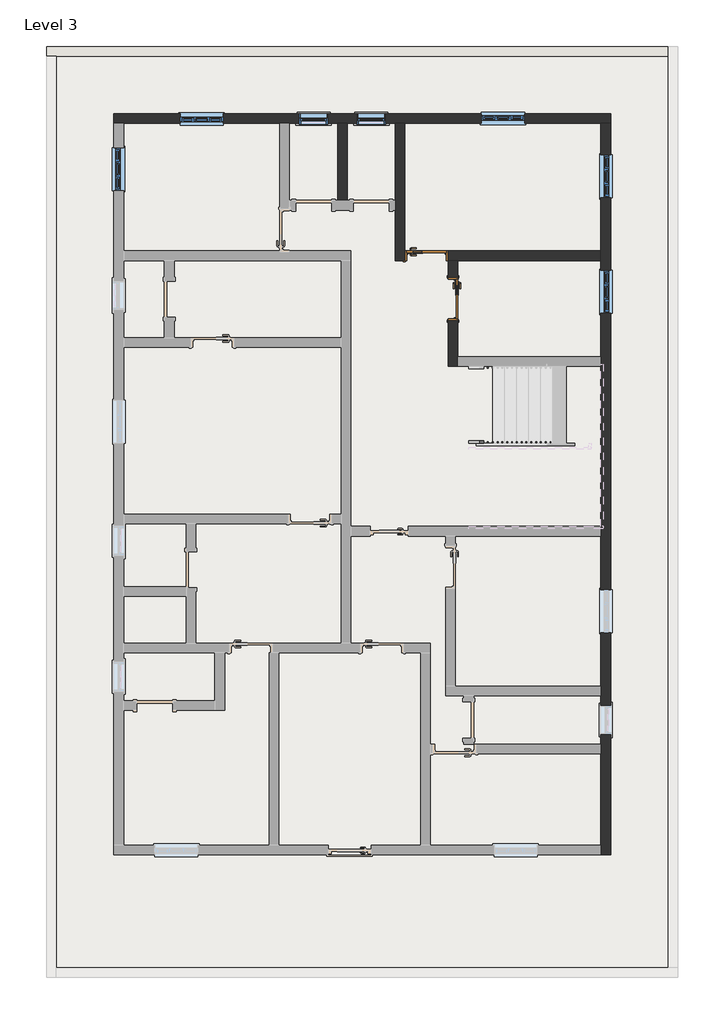
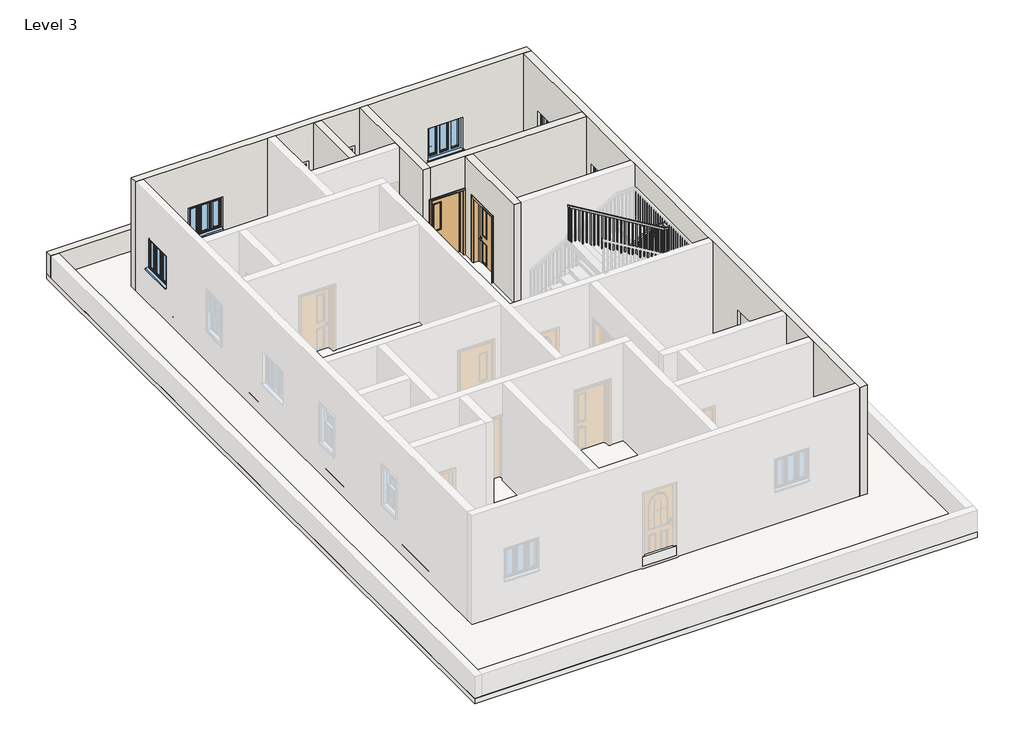
# One storey, part 2 of 3: 7 walls, 7 windows, 2 doors, 2 slabs, 1 railing, 1 roof.
"""IFC4 building model written with IfcOpenShell, lengths in millimetres."""

from ifc_helpers import new_model, si_unit, frame, origin, place, context, project, spatial, polyline, outline, extrude, faceted_brep, transform, mapped, element, save
from components import door_aa1d4bf3, window_679d2811, windows_tpl_w_glazing_bars_910x910mm_9d987a72

model = new_model("IFC4")

# Units and contexts
model_context = context("Model", 3, world=origin())
ifc_project = project(units=[si_unit("LENGTHUNIT", "METRE", prefix="MILLI")], contexts=[model_context])

# Site, building, storey
site = spatial("IfcSite", under=ifc_project)
building = spatial("IfcBuilding", under=site)
storey = spatial("IfcBuildingStorey", under=building, Name="Level 3", Elevation=6096.0)

# Doors
placement = place(None, origin())
door_shape = door_aa1d4bf3(model_context)
element("IfcDoor", 1, ObjectType="Doors_IntSgl_3 : 7'-3\"", at=placement, inside=storey, context=model_context, shape_type="MappedRepresentation", body=[
    mapped(door_shape, transform((-7303.1711241, 14069.3344295, 6096.0), x_axis=(1.0, 0.0, 0.0), y_axis=(0.0, 1.0, 0.0), z_axis=(0.0, 0.0, 1.0))),
])
element("IfcDoor", 2, ObjectType="Doors_IntSgl_3 : 7'-3\"", at=placement, inside=storey, context=model_context, shape_type="MappedRepresentation", body=[
    mapped(door_shape, transform((-6744.3711241, 13154.9344295, 6096.0), x_axis=(0.0, -1.0, 0.0), y_axis=(1.0, 0.0, 0.0), z_axis=(0.0, 0.0, 1.0))),
])

# Railing
element("IfcRailing", 3, ObjectType="Handrail - Rectangular", at=placement, inside=storey, context=model_context, shape_type="SolidModel", body=[
    faceted_brep([(-6414.1711241, 10157.7344295, 7162.8), (-6414.1711241, 10157.7344295, 7103.5575287), (-6414.1711241, 10106.9344295, 7103.5575287), (-6414.1711241, 10106.9344295, 7162.8), (-4128.1711241, 10157.7344295, 8534.4), (-4114.1003386, 10157.7344295, 8483.6), (-4114.1003386, 10106.9344295, 8483.6), (-4128.1711241, 10106.9344295, 8534.4), (-3772.5711241, 10157.7344295, 8534.4), (-3772.5711241, 10157.7344295, 8483.6), (-3823.3711241, 10106.9344295, 8483.6), (-3823.3711241, 10106.9344295, 8534.4), (-3772.5711241, 9929.1344295, 8534.4), (-3772.5711241, 9929.1344295, 8483.6), (-3823.3711241, 9979.9344295, 8483.6), (-3823.3711241, 9979.9344295, 8534.4), (-3874.1711241, 9929.1344295, 8534.4), (-3888.2419095, 9929.1344295, 8483.6), (-3888.2419095, 9979.9344295, 8483.6), (-3874.1711241, 9979.9344295, 8534.4), (-6414.1711241, 9929.1344295, 10058.4), (-6414.1711241, 9979.9344295, 10058.4), (-6414.1711241, 9979.9344295, 9999.1575287), (-6414.1711241, 9929.1344295, 9999.1575287)], [[[0, 1, 2, 3]], [[1, 0, 4, 5]], [[2, 1, 5, 6]], [[3, 2, 6, 7]], [[0, 3, 7, 4]], [[5, 4, 8, 9]], [[6, 5, 9, 10]], [[7, 6, 10, 11]], [[4, 7, 11, 8]], [[9, 8, 12, 13]], [[10, 9, 13, 14]], [[11, 10, 14, 15]], [[8, 11, 15, 12]], [[13, 12, 16, 17]], [[14, 13, 17, 18]], [[15, 14, 18, 19]], [[12, 15, 19, 16]], [[20, 21, 22, 23]], [[17, 16, 20, 23]], [[18, 17, 23, 22]], [[19, 18, 22, 21]], [[16, 19, 21, 20]]]),
    extrude(outline(polyline([(9947.7225287, -6328.4461241), (9959.1525287, -6347.4961241), (8991.6, -6347.4961241), (8991.6, -6328.4461241), (9947.7225287, -6328.4461241)])), frame((0.0, 9945.0094295, 0.0), z_axis=(0.0, 1.0, 0.0), x_axis=(0.0, 0.0, 1.0)), (0.0, 0.0, 1.0), 19.05),
    extrude(outline(polyline([(9886.7625287, -6226.8461241), (9898.1925287, -6245.8961241), (8991.6, -6245.8961241), (8991.6, -6226.8461241), (9886.7625287, -6226.8461241)])), frame((0.0, 9945.0094295, 0.0), z_axis=(0.0, 1.0, 0.0), x_axis=(0.0, 0.0, 1.0)), (0.0, 0.0, 1.0), 19.05),
    extrude(outline(polyline([(9825.8025287, -6125.2461241), (9837.2325287, -6144.2961241), (8839.2, -6144.2961241), (8839.2, -6125.2461241), (9825.8025287, -6125.2461241)])), frame((0.0, 9945.0094295, 0.0), z_axis=(0.0, 1.0, 0.0), x_axis=(0.0, 0.0, 1.0)), (0.0, 0.0, 1.0), 19.05),
    extrude(outline(polyline([(9764.8425287, -6023.6461241), (9776.2725287, -6042.6961241), (8839.2, -6042.6961241), (8839.2, -6023.6461241), (9764.8425287, -6023.6461241)])), frame((0.0, 9945.0094295, 0.0), z_axis=(0.0, 1.0, 0.0), x_axis=(0.0, 0.0, 1.0)), (0.0, 0.0, 1.0), 19.05),
    extrude(outline(polyline([(9703.8825287, -5922.0461241), (9715.3125287, -5941.0961241), (8839.2, -5941.0961241), (8839.2, -5922.0461241), (9703.8825287, -5922.0461241)])), frame((0.0, 9945.0094295, 0.0), z_axis=(0.0, 1.0, 0.0), x_axis=(0.0, 0.0, 1.0)), (0.0, 0.0, 1.0), 19.05),
    extrude(outline(polyline([(9642.9225287, -5820.4461241), (9654.3525287, -5839.4961241), (8686.8, -5839.4961241), (8686.8, -5820.4461241), (9642.9225287, -5820.4461241)])), frame((0.0, 9945.0094295, 0.0), z_axis=(0.0, 1.0, 0.0), x_axis=(0.0, 0.0, 1.0)), (0.0, 0.0, 1.0), 19.05),
    extrude(outline(polyline([(9581.9625287, -5718.8461241), (9593.3925287, -5737.8961241), (8686.8, -5737.8961241), (8686.8, -5718.8461241), (9581.9625287, -5718.8461241)])), frame((0.0, 9945.0094295, 0.0), z_axis=(0.0, 1.0, 0.0), x_axis=(0.0, 0.0, 1.0)), (0.0, 0.0, 1.0), 19.05),
    extrude(outline(polyline([(9521.0025287, -5617.2461241), (9532.4325287, -5636.2961241), (8534.4, -5636.2961241), (8534.4, -5617.2461241), (9521.0025287, -5617.2461241)])), frame((0.0, 9945.0094295, 0.0), z_axis=(0.0, 1.0, 0.0), x_axis=(0.0, 0.0, 1.0)), (0.0, 0.0, 1.0), 19.05),
    extrude(outline(polyline([(9460.0425287, -5515.6461241), (9471.4725287, -5534.6961241), (8534.4, -5534.6961241), (8534.4, -5515.6461241), (9460.0425287, -5515.6461241)])), frame((0.0, 9945.0094295, 0.0), z_axis=(0.0, 1.0, 0.0), x_axis=(0.0, 0.0, 1.0)), (0.0, 0.0, 1.0), 19.05),
    extrude(outline(polyline([(9399.0825287, -5414.0461241), (9410.5125287, -5433.0961241), (8534.4, -5433.0961241), (8534.4, -5414.0461241), (9399.0825287, -5414.0461241)])), frame((0.0, 9945.0094295, 0.0), z_axis=(0.0, 1.0, 0.0), x_axis=(0.0, 0.0, 1.0)), (0.0, 0.0, 1.0), 19.05),
    extrude(outline(polyline([(9338.1225287, -5312.4461241), (9349.5525287, -5331.4961241), (8382.0, -5331.4961241), (8382.0, -5312.4461241), (9338.1225287, -5312.4461241)])), frame((0.0, 9945.0094295, 0.0), z_axis=(0.0, 1.0, 0.0), x_axis=(0.0, 0.0, 1.0)), (0.0, 0.0, 1.0), 19.05),
    extrude(outline(polyline([(9277.1625287, -5210.8461241), (9288.5925287, -5229.8961241), (8382.0, -5229.8961241), (8382.0, -5210.8461241), (9277.1625287, -5210.8461241)])), frame((0.0, 9945.0094295, 0.0), z_axis=(0.0, 1.0, 0.0), x_axis=(0.0, 0.0, 1.0)), (0.0, 0.0, 1.0), 19.05),
    extrude(outline(polyline([(9216.2025287, -5109.2461241), (9227.6325287, -5128.2961241), (8229.6, -5128.2961241), (8229.6, -5109.2461241), (9216.2025287, -5109.2461241)])), frame((0.0, 9945.0094295, 0.0), z_axis=(0.0, 1.0, 0.0), x_axis=(0.0, 0.0, 1.0)), (0.0, 0.0, 1.0), 19.05),
    extrude(outline(polyline([(9155.2425287, -5007.6461241), (9166.6725287, -5026.6961241), (8229.6, -5026.6961241), (8229.6, -5007.6461241), (9155.2425287, -5007.6461241)])), frame((0.0, 9945.0094295, 0.0), z_axis=(0.0, 1.0, 0.0), x_axis=(0.0, 0.0, 1.0)), (0.0, 0.0, 1.0), 19.05),
    extrude(outline(polyline([(9094.2825287, -4906.0461241), (9105.7125287, -4925.0961241), (8229.6, -4925.0961241), (8229.6, -4906.0461241), (9094.2825287, -4906.0461241)])), frame((0.0, 9945.0094295, 0.0), z_axis=(0.0, 1.0, 0.0), x_axis=(0.0, 0.0, 1.0)), (0.0, 0.0, 1.0), 19.05),
    extrude(outline(polyline([(9033.3225287, -4804.4461241), (9044.7525287, -4823.4961241), (8077.2, -4823.4961241), (8077.2, -4804.4461241), (9033.3225287, -4804.4461241)])), frame((0.0, 9945.0094295, 0.0), z_axis=(0.0, 1.0, 0.0), x_axis=(0.0, 0.0, 1.0)), (0.0, 0.0, 1.0), 19.05),
    extrude(outline(polyline([(8972.3625287, -4702.8461241), (8983.7925287, -4721.8961241), (8077.2, -4721.8961241), (8077.2, -4702.8461241), (8972.3625287, -4702.8461241)])), frame((0.0, 9945.0094295, 0.0), z_axis=(0.0, 1.0, 0.0), x_axis=(0.0, 0.0, 1.0)), (0.0, 0.0, 1.0), 19.05),
    extrude(outline(polyline([(8911.4025287, -4601.2461241), (8922.8325287, -4620.2961241), (7924.8, -4620.2961241), (7924.8, -4601.2461241), (8911.4025287, -4601.2461241)])), frame((0.0, 9945.0094295, 0.0), z_axis=(0.0, 1.0, 0.0), x_axis=(0.0, 0.0, 1.0)), (0.0, 0.0, 1.0), 19.05),
    extrude(outline(polyline([(8850.4425287, -4499.6461241), (8861.8725287, -4518.6961241), (7924.8, -4518.6961241), (7924.8, -4499.6461241), (8850.4425287, -4499.6461241)])), frame((0.0, 9945.0094295, 0.0), z_axis=(0.0, 1.0, 0.0), x_axis=(0.0, 0.0, 1.0)), (0.0, 0.0, 1.0), 19.05),
    extrude(outline(polyline([(8789.4825287, -4398.0461241), (8800.9125287, -4417.0961241), (7924.8, -4417.0961241), (7924.8, -4398.0461241), (8789.4825287, -4398.0461241)])), frame((0.0, 9945.0094295, 0.0), z_axis=(0.0, 1.0, 0.0), x_axis=(0.0, 0.0, 1.0)), (0.0, 0.0, 1.0), 19.05),
    extrude(outline(polyline([(8728.5225287, -4296.4461241), (8739.9525287, -4315.4961241), (7772.4, -4315.4961241), (7772.4, -4296.4461241), (8728.5225287, -4296.4461241)])), frame((0.0, 9945.0094295, 0.0), z_axis=(0.0, 1.0, 0.0), x_axis=(0.0, 0.0, 1.0)), (0.0, 0.0, 1.0), 19.05),
    extrude(outline(polyline([(8667.5625287, -4194.8461241), (8678.9925287, -4213.8961241), (7772.4, -4213.8961241), (7772.4, -4194.8461241), (8667.5625287, -4194.8461241)])), frame((0.0, 9945.0094295, 0.0), z_axis=(0.0, 1.0, 0.0), x_axis=(0.0, 0.0, 1.0)), (0.0, 0.0, 1.0), 19.05),
    extrude(outline(polyline([(8606.6025287, -4093.2461241), (8618.0325287, -4112.2961241), (7620.0, -4112.2961241), (7620.0, -4093.2461241), (8606.6025287, -4093.2461241)])), frame((0.0, 9945.0094295, 0.0), z_axis=(0.0, 1.0, 0.0), x_axis=(0.0, 0.0, 1.0)), (0.0, 0.0, 1.0), 19.05),
    extrude(outline(polyline([(8545.6425287, -3991.6461241), (8557.0725287, -4010.6961241), (7620.0, -4010.6961241), (7620.0, -3991.6461241), (8545.6425287, -3991.6461241)])), frame((0.0, 9945.0094295, 0.0), z_axis=(0.0, 1.0, 0.0), x_axis=(0.0, 0.0, 1.0)), (0.0, 0.0, 1.0), 19.05),
    extrude(outline(polyline([(8484.6825287, -3890.0461241), (8496.1125287, -3909.0961241), (7620.0, -3909.0961241), (7620.0, -3890.0461241), (8484.6825287, -3890.0461241)])), frame((0.0, 9945.0094295, 0.0), z_axis=(0.0, 1.0, 0.0), x_axis=(0.0, 0.0, 1.0)), (0.0, 0.0, 1.0), 19.05),
    extrude(outline(polyline([(-3807.4961241, 10040.2594295), (-3788.4461241, 10040.2594295), (-3788.4461241, 10021.2094295), (-3807.4961241, 10021.2094295), (-3807.4961241, 10040.2594295)])), frame((0.0, 0.0, 7620.0), z_axis=(0.0, 0.0, 1.0), x_axis=(1.0, 0.0, 0.0)), (0.0, 0.0, 1.0), 863.6),
    extrude(outline(polyline([(-3883.6961241, 10122.8094295), (-3883.6961241, 10141.8594295), (-3864.6461241, 10141.8594295), (-3864.6461241, 10122.8094295), (-3883.6961241, 10122.8094295)])), frame((0.0, 0.0, 7620.0), z_axis=(0.0, 0.0, 1.0), x_axis=(1.0, 0.0, 0.0)), (0.0, 0.0, 1.0), 863.6),
    extrude(outline(polyline([(-3985.2961241, 10122.8094295), (-3985.2961241, 10141.8594295), (-3966.2461241, 10141.8594295), (-3966.2461241, 10122.8094295), (-3985.2961241, 10122.8094295)])), frame((0.0, 0.0, 7620.0), z_axis=(0.0, 0.0, 1.0), x_axis=(1.0, 0.0, 0.0)), (0.0, 0.0, 1.0), 863.6),
    extrude(outline(polyline([(-4086.8961241, 10122.8094295), (-4086.8961241, 10141.8594295), (-4067.8461241, 10141.8594295), (-4067.8461241, 10122.8094295), (-4086.8961241, 10122.8094295)])), frame((0.0, 0.0, 7620.0), z_axis=(0.0, 0.0, 1.0), x_axis=(1.0, 0.0, 0.0)), (0.0, 0.0, 1.0), 863.6),
    extrude(outline(polyline([(8450.3925287, -4169.4461241), (8438.9625287, -4188.4961241), (7467.6, -4188.4961241), (7467.6, -4169.4461241), (8450.3925287, -4169.4461241)])), frame((0.0, 10122.8094295, 0.0), z_axis=(0.0, 1.0, 0.0), x_axis=(0.0, 0.0, 1.0)), (0.0, 0.0, 1.0), 19.05),
    extrude(outline(polyline([(8389.4325287, -4271.0461241), (8378.0025287, -4290.0961241), (7467.6, -4290.0961241), (7467.6, -4271.0461241), (8389.4325287, -4271.0461241)])), frame((0.0, 10122.8094295, 0.0), z_axis=(0.0, 1.0, 0.0), x_axis=(0.0, 0.0, 1.0)), (0.0, 0.0, 1.0), 19.05),
    extrude(outline(polyline([(8328.4725287, -4372.6461241), (8317.0425287, -4391.6961241), (7467.6, -4391.6961241), (7467.6, -4372.6461241), (8328.4725287, -4372.6461241)])), frame((0.0, 10122.8094295, 0.0), z_axis=(0.0, 1.0, 0.0), x_axis=(0.0, 0.0, 1.0)), (0.0, 0.0, 1.0), 19.05),
    extrude(outline(polyline([(8267.5125287, -4474.2461241), (8256.0825287, -4493.2961241), (7315.2, -4493.2961241), (7315.2, -4474.2461241), (8267.5125287, -4474.2461241)])), frame((0.0, 10122.8094295, 0.0), z_axis=(0.0, 1.0, 0.0), x_axis=(0.0, 0.0, 1.0)), (0.0, 0.0, 1.0), 19.05),
    extrude(outline(polyline([(8206.5525287, -4575.8461241), (8195.1225287, -4594.8961241), (7315.2, -4594.8961241), (7315.2, -4575.8461241), (8206.5525287, -4575.8461241)])), frame((0.0, 10122.8094295, 0.0), z_axis=(0.0, 1.0, 0.0), x_axis=(0.0, 0.0, 1.0)), (0.0, 0.0, 1.0), 19.05),
    extrude(outline(polyline([(8145.5925287, -4677.4461241), (8134.1625287, -4696.4961241), (7162.8, -4696.4961241), (7162.8, -4677.4461241), (8145.5925287, -4677.4461241)])), frame((0.0, 10122.8094295, 0.0), z_axis=(0.0, 1.0, 0.0), x_axis=(0.0, 0.0, 1.0)), (0.0, 0.0, 1.0), 19.05),
    extrude(outline(polyline([(8084.6325287, -4779.0461241), (8073.2025287, -4798.0961241), (7162.8, -4798.0961241), (7162.8, -4779.0461241), (8084.6325287, -4779.0461241)])), frame((0.0, 10122.8094295, 0.0), z_axis=(0.0, 1.0, 0.0), x_axis=(0.0, 0.0, 1.0)), (0.0, 0.0, 1.0), 19.05),
    extrude(outline(polyline([(8023.6725287, -4880.6461241), (8012.2425287, -4899.6961241), (7162.8, -4899.6961241), (7162.8, -4880.6461241), (8023.6725287, -4880.6461241)])), frame((0.0, 10122.8094295, 0.0), z_axis=(0.0, 1.0, 0.0), x_axis=(0.0, 0.0, 1.0)), (0.0, 0.0, 1.0), 19.05),
    extrude(outline(polyline([(7962.7125287, -4982.2461241), (7951.2825287, -5001.2961241), (7010.4, -5001.2961241), (7010.4, -4982.2461241), (7962.7125287, -4982.2461241)])), frame((0.0, 10122.8094295, 0.0), z_axis=(0.0, 1.0, 0.0), x_axis=(0.0, 0.0, 1.0)), (0.0, 0.0, 1.0), 19.05),
    extrude(outline(polyline([(7901.7525287, -5083.8461241), (7890.3225287, -5102.8961241), (7010.4, -5102.8961241), (7010.4, -5083.8461241), (7901.7525287, -5083.8461241)])), frame((0.0, 10122.8094295, 0.0), z_axis=(0.0, 1.0, 0.0), x_axis=(0.0, 0.0, 1.0)), (0.0, 0.0, 1.0), 19.05),
    extrude(outline(polyline([(7840.7925287, -5185.4461241), (7829.3625287, -5204.4961241), (6858.0, -5204.4961241), (6858.0, -5185.4461241), (7840.7925287, -5185.4461241)])), frame((0.0, 10122.8094295, 0.0), z_axis=(0.0, 1.0, 0.0), x_axis=(0.0, 0.0, 1.0)), (0.0, 0.0, 1.0), 19.05),
    extrude(outline(polyline([(7779.8325287, -5287.0461241), (7768.4025287, -5306.0961241), (6858.0, -5306.0961241), (6858.0, -5287.0461241), (7779.8325287, -5287.0461241)])), frame((0.0, 10122.8094295, 0.0), z_axis=(0.0, 1.0, 0.0), x_axis=(0.0, 0.0, 1.0)), (0.0, 0.0, 1.0), 19.05),
    extrude(outline(polyline([(7718.8725287, -5388.6461241), (7707.4425287, -5407.6961241), (6858.0, -5407.6961241), (6858.0, -5388.6461241), (7718.8725287, -5388.6461241)])), frame((0.0, 10122.8094295, 0.0), z_axis=(0.0, 1.0, 0.0), x_axis=(0.0, 0.0, 1.0)), (0.0, 0.0, 1.0), 19.05),
    extrude(outline(polyline([(7657.9125287, -5490.2461241), (7646.4825287, -5509.2961241), (6705.6, -5509.2961241), (6705.6, -5490.2461241), (7657.9125287, -5490.2461241)])), frame((0.0, 10122.8094295, 0.0), z_axis=(0.0, 1.0, 0.0), x_axis=(0.0, 0.0, 1.0)), (0.0, 0.0, 1.0), 19.05),
    extrude(outline(polyline([(7596.9525287, -5591.8461241), (7585.5225287, -5610.8961241), (6705.6, -5610.8961241), (6705.6, -5591.8461241), (7596.9525287, -5591.8461241)])), frame((0.0, 10122.8094295, 0.0), z_axis=(0.0, 1.0, 0.0), x_axis=(0.0, 0.0, 1.0)), (0.0, 0.0, 1.0), 19.05),
    extrude(outline(polyline([(7535.9925287, -5693.4461241), (7524.5625287, -5712.4961241), (6553.2, -5712.4961241), (6553.2, -5693.4461241), (7535.9925287, -5693.4461241)])), frame((0.0, 10122.8094295, 0.0), z_axis=(0.0, 1.0, 0.0), x_axis=(0.0, 0.0, 1.0)), (0.0, 0.0, 1.0), 19.05),
    extrude(outline(polyline([(7475.0325287, -5795.0461241), (7463.6025287, -5814.0961241), (6553.2, -5814.0961241), (6553.2, -5795.0461241), (7475.0325287, -5795.0461241)])), frame((0.0, 10122.8094295, 0.0), z_axis=(0.0, 1.0, 0.0), x_axis=(0.0, 0.0, 1.0)), (0.0, 0.0, 1.0), 19.05),
    extrude(outline(polyline([(7414.0725287, -5896.6461241), (7402.6425287, -5915.6961241), (6553.2, -5915.6961241), (6553.2, -5896.6461241), (7414.0725287, -5896.6461241)])), frame((0.0, 10122.8094295, 0.0), z_axis=(0.0, 1.0, 0.0), x_axis=(0.0, 0.0, 1.0)), (0.0, 0.0, 1.0), 19.05),
    extrude(outline(polyline([(7353.1125287, -5998.2461241), (7341.6825287, -6017.2961241), (6400.8, -6017.2961241), (6400.8, -5998.2461241), (7353.1125287, -5998.2461241)])), frame((0.0, 10122.8094295, 0.0), z_axis=(0.0, 1.0, 0.0), x_axis=(0.0, 0.0, 1.0)), (0.0, 0.0, 1.0), 19.05),
    extrude(outline(polyline([(7292.1525287, -6099.8461241), (7280.7225287, -6118.8961241), (6400.8, -6118.8961241), (6400.8, -6099.8461241), (7292.1525287, -6099.8461241)])), frame((0.0, 10122.8094295, 0.0), z_axis=(0.0, 1.0, 0.0), x_axis=(0.0, 0.0, 1.0)), (0.0, 0.0, 1.0), 19.05),
    extrude(outline(polyline([(7231.1925287, -6201.4461241), (7219.7625287, -6220.4961241), (6248.4, -6220.4961241), (6248.4, -6201.4461241), (7231.1925287, -6201.4461241)])), frame((0.0, 10122.8094295, 0.0), z_axis=(0.0, 1.0, 0.0), x_axis=(0.0, 0.0, 1.0)), (0.0, 0.0, 1.0), 19.05),
    extrude(outline(polyline([(7170.2325287, -6303.0461241), (7158.8025287, -6322.0961241), (6248.4, -6322.0961241), (6248.4, -6303.0461241), (7170.2325287, -6303.0461241)])), frame((0.0, 10122.8094295, 0.0), z_axis=(0.0, 1.0, 0.0), x_axis=(0.0, 0.0, 1.0)), (0.0, 0.0, 1.0), 19.05),
    extrude(outline(polyline([(-3807.4961241, 9964.0594295), (-3788.4461241, 9964.0594295), (-3788.4461241, 9945.0094295), (-3807.4961241, 9945.0094295), (-3807.4961241, 9964.0594295)])), frame((0.0, 0.0, 7620.0), z_axis=(0.0, 0.0, 1.0), x_axis=(1.0, 0.0, 0.0)), (0.0, 0.0, 1.0), 863.6),
    extrude(outline(polyline([(-3807.4961241, 10122.8094295), (-3807.4961241, 10141.8594295), (-3788.4461241, 10141.8594295), (-3788.4461241, 10122.8094295), (-3807.4961241, 10122.8094295)])), frame((0.0, 0.0, 7620.0), z_axis=(0.0, 0.0, 1.0), x_axis=(1.0, 0.0, 0.0)), (0.0, 0.0, 1.0), 863.6),
    extrude(outline(polyline([(9987.7275287, -6395.1211241), (9999.1575287, -6414.1711241), (8991.6, -6414.1711241), (8991.6, -6395.1211241), (9987.7275287, -6395.1211241)])), frame((0.0, 9945.0094295, 0.0), z_axis=(0.0, 1.0, 0.0), x_axis=(0.0, 0.0, 1.0)), (0.0, 0.0, 1.0), 19.05),
    extrude(outline(polyline([(7114.9875287, -6395.1211241), (7103.5575287, -6414.1711241), (6248.4, -6414.1711241), (6248.4, -6395.1211241), (7114.9875287, -6395.1211241)])), frame((0.0, 10122.8094295, 0.0), z_axis=(0.0, 1.0, 0.0), x_axis=(0.0, 0.0, 1.0)), (0.0, 0.0, 1.0), 19.05),
])

# Roof
element("IfcRoof", 4, ObjectType="Generic - 12\"", at=placement, inside=storey, context=model_context, shape_type="SweptSolid", body=[
    extrude(outline(polyline([(-13907.1711241, 17066.5344295), (-3416.9711241, 17066.5344295), (-3416.9711241, 1420.1344295), (-13907.1711241, 1420.1344295), (-13907.1711241, 17066.5344295)])), frame((0.0, 0.0, 6096.0), z_axis=(0.0, 0.0, 1.0), x_axis=(1.0, 0.0, 0.0)), (0.0, 0.0, 1.0), 304.8),
])

# Slabs
element("IfcSlab", 5, ObjectType="Generic - 12\"", at=placement, inside=storey, context=model_context, shape_type="SweptSolid", body=[
    extrude(outline(polyline([(-1994.5711241, 18488.2009778), (-1994.5711241, -1171.3990222), (-15329.5711241, -1171.3990222), (-15329.5711241, 18488.2009778), (-1994.5711241, 18488.2009778)])), frame((0.0, 0.0, 5943.6), z_axis=(0.0, 0.0, 1.0), x_axis=(1.0, 0.0, 0.0)), (0.0, 0.0, 1.0), 152.4),
])
element("IfcSlab", 6, ObjectType="Generic - 12\" 2", at=placement, inside=storey, context=model_context, shape_type="SweptSolid", body=[
    extrude(outline(polyline([(-3416.9711241, 17066.5344295), (-3416.9711241, 1420.1344295), (-13907.1711241, 1420.1344295), (-13907.1711241, 17066.5344295), (-3416.9711241, 17066.5344295)])), frame((0.0, 0.0, 5943.6), z_axis=(0.0, 0.0, 1.0), x_axis=(1.0, 0.0, 0.0)), (0.0, 0.0, 1.0), 152.4),
])

# Walls
element("IfcWall", 7, ObjectType="Generic -4.5\" p", at=placement, inside=storey, context=model_context, shape_type="SweptSolid", body=[
    extrude(outline(polyline([(-9182.7711241, 15237.7344295), (-9182.7711241, 16863.3344295), (-8979.5711241, 16863.3344295), (-8979.5711241, 15237.7344295), (-9182.7711241, 15237.7344295)])), frame((0.0, 0.0, 6096.0), z_axis=(0.0, 0.0, 1.0), x_axis=(1.0, 0.0, 0.0)), (0.0, 0.0, 1.0), 3048.0),
])
element("IfcWall", 8, ObjectType="Generic -4.5\" p", at=placement, inside=storey, context=model_context, shape_type="Brep", body=[
    faceted_brep([(-7963.5711241, 16863.3344295, 6096.0), (-7963.5711241, 15237.7344295, 6096.0), (-7963.5711241, 15034.5344295, 6096.0), (-7963.5711241, 13967.7344295, 6096.0), (-7963.5711241, 13967.7344295, 9144.0), (-7963.5711241, 15034.5344295, 9144.0), (-7963.5711241, 15237.7344295, 9144.0), (-7963.5711241, 16863.3344295, 9144.0), (-7760.3711241, 16863.3344295, 6096.0), (-7760.3711241, 16863.3344295, 9144.0), (-7760.3711241, 14170.9344295, 9144.0), (-7760.3711241, 13967.7344295, 9144.0), (-7760.3711241, 13967.7344295, 8229.6), (-7760.3711241, 13967.7344295, 6096.0)], [[[0, 1, 2, 3, 4, 5, 6, 7]], [[8, 9, 10, 11, 12, 13]], [[3, 2, 1, 0, 8, 13]], [[7, 6, 5, 4, 11, 10, 9]], [[0, 7, 9, 8]], [[4, 3, 13, 12, 11]]]),
])
element("IfcWall", 9, ObjectType="Generic -4.5\" p", at=placement, inside=storey, context=model_context, shape_type="Brep", body=[
    faceted_brep([(-7760.3711241, 14170.9344295, 9144.0), (-3620.1711241, 14170.9344295, 9144.0), (-3620.1711241, 14170.9344295, 6096.0), (-6845.9711241, 14170.9344295, 6096.0), (-6845.9711241, 14170.9344295, 8229.6), (-7760.3711241, 14170.9344295, 8229.6), (-3620.1711241, 13967.7344295, 9144.0), (-6642.7711241, 13967.7344295, 9144.0), (-6845.9711241, 13967.7344295, 9144.0), (-7760.3711241, 13967.7344295, 9144.0), (-7760.3711241, 13967.7344295, 8229.6), (-6845.9711241, 13967.7344295, 8229.6), (-6845.9711241, 13967.7344295, 6096.0), (-6642.7711241, 13967.7344295, 6096.0), (-3620.1711241, 13967.7344295, 6096.0)], [[[0, 1, 2, 3, 4, 5]], [[6, 7, 8, 9, 10, 11, 12, 13, 14]], [[2, 14, 13, 12, 3]], [[1, 0, 9, 8, 7, 6]], [[9, 0, 5, 10]], [[2, 1, 6, 14]], [[11, 4, 3, 12]], [[4, 11, 10, 5]]]),
])
element("IfcWall", 10, ObjectType="Generic -4.5\" p", at=placement, inside=storey, context=model_context, shape_type="Brep", body=[
    faceted_brep([(-6845.9711241, 11732.5344295, 9144.0), (-6845.9711241, 13967.7344295, 9144.0), (-6845.9711241, 13967.7344295, 8229.6), (-6845.9711241, 13967.7344295, 6096.0), (-6845.9711241, 13612.1344295, 6096.0), (-6845.9711241, 13612.1344295, 8229.6), (-6845.9711241, 12697.7344295, 8229.6), (-6845.9711241, 12697.7344295, 6096.0), (-6845.9711241, 11732.5344295, 6096.0), (-6642.7711241, 13967.7344295, 9144.0), (-6642.7711241, 11935.7344295, 9144.0), (-6642.7711241, 11732.5344295, 9144.0), (-6642.7711241, 11732.5344295, 6096.0), (-6642.7711241, 11935.7344295, 6096.0), (-6642.7711241, 12697.7344295, 6096.0), (-6642.7711241, 12697.7344295, 8229.6), (-6642.7711241, 13612.1344295, 8229.6), (-6642.7711241, 13612.1344295, 6096.0), (-6642.7711241, 13967.7344295, 6096.0)], [[[0, 1, 2, 3, 4, 5, 6, 7, 8]], [[9, 10, 11, 12, 13, 14, 15, 16, 17, 18]], [[3, 18, 17, 4]], [[12, 8, 7, 14, 13]], [[1, 0, 11, 10, 9]], [[3, 2, 1, 9, 18]], [[0, 8, 12, 11]], [[6, 15, 14, 7]], [[15, 6, 5, 16]], [[16, 5, 4, 17]]]),
])
element("IfcWall", 11, ObjectType="Generic -4.5\" p", at=placement, inside=storey, context=model_context, shape_type="Brep", body=[
    faceted_brep([(-15329.5711241, 18285.0009778, 6096.0), (-15126.3711241, 18285.0009778, 6096.0), (-2197.7711241, 18285.0009778, 6096.0), (-2197.7711241, 18285.0009778, 6705.6), (-15126.3711241, 18285.0009778, 6705.6), (-15329.5711241, 18285.0009778, 6705.6), (-15329.5711241, 18488.2009778, 6096.0), (-15329.5711241, 18488.2009778, 6705.6), (-2197.7711241, 18488.2009778, 6705.6), (-2197.7711241, 18488.2009778, 6096.0)], [[[0, 1, 2, 3, 4, 5]], [[6, 7, 8, 9]], [[2, 1, 0, 6, 9]], [[5, 4, 3, 8, 7]], [[0, 5, 7, 6]], [[3, 2, 9, 8]]]),
])
element("IfcWall", 12, ObjectType="Generic -9\" w", at=placement, inside=storey, context=model_context, shape_type="Brep", body=[
    faceted_brep([(-13907.1711241, 16863.3344295, 6096.0), (-13703.9711241, 16863.3344295, 6096.0), (-10401.9711241, 16863.3344295, 6096.0), (-10198.7711241, 16863.3344295, 6096.0), (-9182.7711241, 16863.3344295, 6096.0), (-8979.5711241, 16863.3344295, 6096.0), (-7963.5711241, 16863.3344295, 6096.0), (-7760.3711241, 16863.3344295, 6096.0), (-3620.1711241, 16863.3344295, 6096.0), (-3416.9711241, 16863.3344295, 6096.0), (-3416.9711241, 16863.3344295, 9144.0), (-3620.1711241, 16863.3344295, 9144.0), (-7760.3711241, 16863.3344295, 9144.0), (-7963.5711241, 16863.3344295, 9144.0), (-8979.5711241, 16863.3344295, 9144.0), (-9182.7711241, 16863.3344295, 9144.0), (-10198.7711241, 16863.3344295, 9144.0), (-10401.9711241, 16863.3344295, 9144.0), (-13703.9711241, 16863.3344295, 9144.0), (-13907.1711241, 16863.3344295, 9144.0), (-11597.9711241, 16863.3344295, 7920.4), (-11597.9711241, 16863.3344295, 7010.4), (-12507.9711241, 16863.3344295, 7010.4), (-12507.9711241, 16863.3344295, 7920.4), (-6145.2711241, 16863.3344295, 7920.4), (-5235.2711241, 16863.3344295, 7920.4), (-5235.2711241, 16863.3344295, 7010.4), (-6145.2711241, 16863.3344295, 7010.4), (-9385.9711241, 16863.3344295, 8077.2), (-9385.9711241, 16863.3344295, 7010.4), (-9995.5711241, 16863.3344295, 7010.4), (-9995.5711241, 16863.3344295, 8077.2), (-8166.7711241, 16863.3344295, 8077.2), (-8166.7711241, 16863.3344295, 7010.4), (-8776.3711241, 16863.3344295, 7010.4), (-8776.3711241, 16863.3344295, 8077.2), (-13907.1711241, 17066.5344295, 6096.0), (-13907.1711241, 17066.5344295, 9144.0), (-3416.9711241, 17066.5344295, 9144.0), (-3416.9711241, 17066.5344295, 6096.0), (-11597.9711241, 17066.5344295, 7920.4), (-12507.9711241, 17066.5344295, 7920.4), (-12507.9711241, 17066.5344295, 7010.4), (-11597.9711241, 17066.5344295, 7010.4), (-6145.2711241, 17066.5344295, 7920.4), (-6145.2711241, 17066.5344295, 7010.4), (-5235.2711241, 17066.5344295, 7010.4), (-5235.2711241, 17066.5344295, 7920.4), (-9385.9711241, 17066.5344295, 8077.2), (-9995.5711241, 17066.5344295, 8077.2), (-9995.5711241, 17066.5344295, 7010.4), (-9385.9711241, 17066.5344295, 7010.4), (-8166.7711241, 17066.5344295, 8077.2), (-8776.3711241, 17066.5344295, 8077.2), (-8776.3711241, 17066.5344295, 7010.4), (-8166.7711241, 17066.5344295, 7010.4)], [[[0, 1, 2, 3, 4, 5, 6, 7, 8, 9, 10, 11, 12, 13, 14, 15, 16, 17, 18, 19], [20, 21, 22, 23], [24, 25, 26, 27], [28, 29, 30, 31], [32, 33, 34, 35]], [[36, 37, 38, 39], [40, 41, 42, 43], [44, 45, 46, 47], [48, 49, 50, 51], [52, 53, 54, 55]], [[9, 8, 7, 6, 5, 4, 3, 2, 1, 0, 36, 39]], [[19, 18, 17, 16, 15, 14, 13, 12, 11, 10, 38, 37]], [[10, 9, 39, 38]], [[0, 19, 37, 36]], [[21, 20, 40, 43]], [[22, 21, 43, 42]], [[23, 22, 42, 41]], [[20, 23, 41, 40]], [[45, 44, 24, 27]], [[46, 45, 27, 26]], [[47, 46, 26, 25]], [[44, 47, 25, 24]], [[29, 28, 48, 51]], [[30, 29, 51, 50]], [[31, 30, 50, 49]], [[28, 31, 49, 48]], [[33, 32, 52, 55]], [[34, 33, 55, 54]], [[35, 34, 54, 53]], [[32, 35, 53, 52]]]),
])
element("IfcWall", 13, ObjectType="Generic -9\" w", at=placement, inside=storey, context=model_context, shape_type="Brep", body=[
    faceted_brep([(-3620.1711241, 16863.3344295, 6096.0), (-3620.1711241, 14170.9344295, 6096.0), (-3620.1711241, 13967.7344295, 6096.0), (-3620.1711241, 11935.7344295, 6096.0), (-3620.1711241, 11732.5344295, 6096.0), (-3620.1711241, 8354.3344295, 6096.0), (-3620.1711241, 8151.1344295, 6096.0), (-3620.1711241, 4976.1344295, 6096.0), (-3620.1711241, 4772.9344295, 6096.0), (-3620.1711241, 3756.9344295, 6096.0), (-3620.1711241, 3553.7344295, 6096.0), (-3620.1711241, 1623.3344295, 6096.0), (-3620.1711241, 1420.1344295, 6096.0), (-3620.1711241, 1420.1344295, 9144.0), (-3620.1711241, 1623.3344295, 9144.0), (-3620.1711241, 3553.7344295, 9144.0), (-3620.1711241, 3756.9344295, 9144.0), (-3620.1711241, 4772.9344295, 9144.0), (-3620.1711241, 4976.1344295, 9144.0), (-3620.1711241, 8151.1344295, 9144.0), (-3620.1711241, 8354.3344295, 9144.0), (-3620.1711241, 11732.5344295, 9144.0), (-3620.1711241, 11935.7344295, 9144.0), (-3620.1711241, 13967.7344295, 9144.0), (-3620.1711241, 14170.9344295, 9144.0), (-3620.1711241, 16863.3344295, 9144.0), (-3620.1711241, 16200.7344295, 7920.4), (-3620.1711241, 15290.7344295, 7920.4), (-3620.1711241, 15290.7344295, 7010.4), (-3620.1711241, 16200.7344295, 7010.4), (-3620.1711241, 13762.3344295, 7920.4), (-3620.1711241, 12852.3344295, 7920.4), (-3620.1711241, 12852.3344295, 7010.4), (-3620.1711241, 13762.3344295, 7010.4), (-3620.1711241, 7018.6344295, 7920.4), (-3620.1711241, 6108.6344295, 7920.4), (-3620.1711241, 6108.6344295, 7010.4), (-3620.1711241, 7018.6344295, 7010.4), (-3620.1711241, 4569.7344295, 8077.2), (-3620.1711241, 3960.1344295, 8077.2), (-3620.1711241, 3960.1344295, 7010.4), (-3620.1711241, 4569.7344295, 7010.4), (-3416.9711241, 16863.3344295, 6096.0), (-3416.9711241, 16863.3344295, 9144.0), (-3416.9711241, 1420.1344295, 9144.0), (-3416.9711241, 1420.1344295, 6096.0), (-3416.9711241, 16200.7344295, 7920.4), (-3416.9711241, 16200.7344295, 7010.4), (-3416.9711241, 15290.7344295, 7010.4), (-3416.9711241, 15290.7344295, 7920.4), (-3416.9711241, 13762.3344295, 7920.4), (-3416.9711241, 13762.3344295, 7010.4), (-3416.9711241, 12852.3344295, 7010.4), (-3416.9711241, 12852.3344295, 7920.4), (-3416.9711241, 7018.6344295, 7920.4), (-3416.9711241, 7018.6344295, 7010.4), (-3416.9711241, 6108.6344295, 7010.4), (-3416.9711241, 6108.6344295, 7920.4), (-3416.9711241, 4569.7344295, 8077.2), (-3416.9711241, 4569.7344295, 7010.4), (-3416.9711241, 3960.1344295, 7010.4), (-3416.9711241, 3960.1344295, 8077.2)], [[[0, 1, 2, 3, 4, 5, 6, 7, 8, 9, 10, 11, 12, 13, 14, 15, 16, 17, 18, 19, 20, 21, 22, 23, 24, 25], [26, 27, 28, 29], [30, 31, 32, 33], [34, 35, 36, 37], [38, 39, 40, 41]], [[42, 43, 44, 45], [46, 47, 48, 49], [50, 51, 52, 53], [54, 55, 56, 57], [58, 59, 60, 61]], [[12, 11, 10, 9, 8, 7, 6, 5, 4, 3, 2, 1, 0, 42, 45]], [[25, 24, 23, 22, 21, 20, 19, 18, 17, 16, 15, 14, 13, 44, 43]], [[0, 25, 43, 42]], [[13, 12, 45, 44]], [[47, 46, 26, 29]], [[48, 47, 29, 28]], [[49, 48, 28, 27]], [[46, 49, 27, 26]], [[51, 50, 30, 33]], [[52, 51, 33, 32]], [[53, 52, 32, 31]], [[50, 53, 31, 30]], [[55, 54, 34, 37]], [[56, 55, 37, 36]], [[57, 56, 36, 35]], [[54, 57, 35, 34]], [[59, 58, 38, 41]], [[60, 59, 41, 40]], [[61, 60, 40, 39]], [[58, 61, 39, 38]]]),
])

# Windows
window_shape = window_679d2811(model_context)
element("IfcWindow", 14, ObjectType="Window-Double-Hung : 24\" x 42\"", at=placement, inside=storey, context=model_context, shape_type="MappedRepresentation", body=[
    mapped(window_shape, transform((-9690.7711241, 16964.9344295, 6096.0), x_axis=(-1.0, 0.0, 0.0), y_axis=(0.0, -1.0, 0.0), z_axis=(0.0, 0.0, 1.0))),
])
element("IfcWindow", 15, ObjectType="Window-Double-Hung : 24\" x 42\"", at=placement, inside=storey, context=model_context, shape_type="MappedRepresentation", body=[
    mapped(window_shape, transform((-8471.5711241, 16964.9344295, 6096.0), x_axis=(-1.0, 0.0, 0.0), y_axis=(0.0, -1.0, 0.0), z_axis=(0.0, 0.0, 1.0))),
])
windows_tpl_w_glazing_bars_910x910mm_shape = windows_tpl_w_glazing_bars_910x910mm_9d987a72(model_context)
element("IfcWindow", 16, ObjectType="Windows_Tpl_w-Glazing_Bars : 910x910mm", at=placement, inside=storey, context=model_context, shape_type="MappedRepresentation", body=[
    mapped(windows_tpl_w_glazing_bars_910x910mm_shape, transform((-12289.6377907, 16973.3909974, 5810.4), x_axis=(-1.0, 0.0, 0.0), y_axis=(0.0, -1.0, 0.0), z_axis=(0.0, 0.0, 1.0))),
])
element("IfcWindow", 17, ObjectType="Windows_Tpl_w-Glazing_Bars : 910x910mm", at=placement, inside=storey, context=model_context, shape_type="MappedRepresentation", body=[
    mapped(windows_tpl_w_glazing_bars_910x910mm_shape, transform((-5453.6044574, 16956.4778617, 5810.4), x_axis=(1.0, 0.0, 0.0), y_axis=(0.0, 1.0, 0.0), z_axis=(0.0, 0.0, 1.0))),
])
element("IfcWindow", 18, ObjectType="Windows_Tpl_w-Glazing_Bars : 910x910mm", at=placement, inside=storey, context=model_context, shape_type="MappedRepresentation", body=[
    mapped(windows_tpl_w_glazing_bars_910x910mm_shape, transform((-3527.0276919, 15509.0677629, 5810.4), x_axis=(0.0, -1.0, 0.0), y_axis=(1.0, 0.0, 0.0), z_axis=(0.0, 0.0, 1.0))),
])
element("IfcWindow", 19, ObjectType="Windows_Tpl_w-Glazing_Bars : 910x910mm", at=placement, inside=storey, context=model_context, shape_type="MappedRepresentation", body=[
    mapped(windows_tpl_w_glazing_bars_910x910mm_shape, transform((-13797.1145562, 16134.8010962, 5810.4), x_axis=(0.0, 1.0, 0.0), y_axis=(-1.0, 0.0, 0.0), z_axis=(0.0, 0.0, 1.0))),
])
element("IfcWindow", 20, ObjectType="Windows_Tpl_w-Glazing_Bars : 910x910mm", at=placement, inside=storey, context=model_context, shape_type="MappedRepresentation", body=[
    mapped(windows_tpl_w_glazing_bars_910x910mm_shape, transform((-3527.0276919, 13070.6677629, 5810.4), x_axis=(0.0, -1.0, 0.0), y_axis=(1.0, 0.0, 0.0), z_axis=(0.0, 0.0, 1.0))),
])

save(model, "model.ifc")

# Revit data of these elements
# Type "Doors_IntSgl_3 : 7'-3\""
#   Type Mark = "14"
#   Type Comments = "Internal Single"
#   Operation = "SingleSwingRight"
#   Construction Type Id = "SGL"
#   Manufacturer = "Revit"
#   Keynote = "L20"
#   Description = "Internal Single Door"
#   Analytic Construction = "Large single-glazed windows"
#   Visual Light Transmittance = 0.9
#   VisionPanel Width = 0' - 7.87402"
#   UnderCut = 0' - 0.31496"
#   Tolerance = 0' - 0.07874"
#   Structural Tolerance = 0' - 0.31496"
#   StopDepth = 0' - 1.25984"
#   Stop Thickness = 0' - 0.74803"
#   Stile Top of Lock Rail = 3' - 7.30709"
#   Stile Top Rail = 0' - 8.85827"
#   Stile Shutting = 0' - 4.92126"
#   Stile Lock Rail = 0' - 6.88976"
#   Stile Bottom Rail = 1' - 1.77953"
#   Solar Heat Gain Coefficient = 0.86
#   Rough Width = 3' - 0"
#   Rough Height = 7' - 0"
#   Heat Transfer Coefficient (U) = 0.979472 BTU/(h·ft²·°F)
#   Handle Z Distance = 3' - 3.37008"
#   Handle X Distance = 0' - 2.95276"
#   Frame Thickness = 0' - 1.25984"
#   Door Panel Width = 2' - 8.69291"
#   Door Panel Thickness = 0' - 1.49606"
#   Door Panel Offset = 0' - 0"
#   Height = 7' - 0"
#   Width = 3' - 0"
#   Door Panel Height = 6' - 10.0315"
#   Architrave Setback = 0' - 0.19685"
#   Vis - Ironmongery = yes
#   Define Thermal Properties by = 1
#   Material Ironmongery = Door - Handle
#   Material Glass = Door - Glazing
#   Material Frame = Door - Frame/Mullion
#   Material Door = Door - Panel
#   Material Beading = Door - Panel
#   Material Architrave = Door - Architrave
#   Function = (empty or 0)
#   Wall Closure = (empty or 0)
# Type "Handrail - Rectangular"
#   Assembly Code = "C2010400"
#   built-in parameter 1008612 = 0.0416667 (stored number, unit not read)
#   built-in parameter 1008611 = 0.0416667 (stored number, unit not read)
#   built-in parameter 1008609 = 0.333333 (stored number, unit not read)
#   built-in parameter 1008604 = 0.166667 (stored number, unit not read)
#   built-in parameter 1008603 = 0.166667 (stored number, unit not read)
#   Railing Height = 3' - 0"
#   built-in parameter 1008630 = 2
#   built-in parameter 1008610 = 2
#   built-in parameter 1008618 = Baluster - Square : 3/4"
# Type "Generic - 12\""
#   Assembly Code = "B1020"
#   Layers, outside or top first: 1' - 0" no material (function 1)
# Type "Generic - 12\""
#   Assembly Code = "B1010"
#   Function = 0
#   Layers, outside or top first: 0' - 6" no material (function 1)
# Type "Generic - 12\" 2"
#   Assembly Code = "B1010"
#   Function = 0
#   Layers, outside or top first: 0' - 6" no material (function 1)
# Type "Generic -4.5\" p"
#   Assembly Code = "B2010"
#   Layers, outside or top first: 0' - 8" no material (function 1)
# Type "Generic -9\" w"
#   Assembly Code = "B2010"
#   Layers, outside or top first: 0' - 8" no material (function 1)
# Type "Window-Double-Hung : 24\" x 42\""
#   Type Mark = "10"
#   Fire Rating = "0.5h"
#   Construction Type Id = "DG-DR"
#   Assembly Code = "B2020100"
#   Analytic Construction = "Double glazing - domestic"
#   Wall Thickness [instance default] = 0' - 6"
#   Window Inset [instance default] = 0' - 0"
#   Visual Light Transmittance = 0.81
#   Thermal Resistance (R) = 1.8146 (h·ft²·°F)/BTU
#   Solar Heat Gain Coefficient = 0.76
#   Muntin Width = 1' - 6"
#   Muntin Height = 1' - 5 1/8"
#   Interior Wall Closure [instance default] = 0' - 1 1/2"
#   Rough Width = 2' - 0 1/2"
#   Rough Height = 3' - 6 1/2"
#   Frame Extension [instance default] = 0' - 1 1/4"
#   Exterior Wall Closure [instance default] = 0' - 0 1/2"
#   Extension Jamb [instance default] = 0' - 1 1/2"
#   Heat Transfer Coefficient (U) = 0.5511 BTU/(h·ft²·°F)
#   Height = 3' - 6"
#   Width = 2' - 0"
#   Define Thermal Properties by = 1
#   Top Muntin Visibility = yes
#   Indicator Visibility [instance default] = yes
#   Extension Jamb Visibility [instance default] = yes
#   Interior Trim Visibility [instance default] = yes
#   Exterior Trim Visibility [instance default] = yes
#   Define Thermal Properties by = 1
#   Bottom Muntin Visibility = yes
#   Muntin Pattern = Muntin Pattern_2x2 : Muntin Pattern_2x2
#   Interior Trim Material = Wood - Stained
#   Interior Trim = Trim-Window-Interior-Flat : Picture Frame
#   Exterior Trim Material = Clad - White
#   Exterior Trim = Trim-Window-Exterior-Flat : with Sill
#   Glass Panel Material = Glass
#   Exterior Frame Material = Clad - White
#   Interior Frame Material = Wood - Stained
#   Wall Closure = (empty or 0)
# Type "Windows_Tpl_w-Glazing_Bars : 910x910mm"
#   Type Mark = "18"
#   Operation = "TriplePanelVertical"
#   Construction Type Id = "GSP4R"
#   Manufacturer = "Revit"
#   Keynote = "L10"
#   Analytic Construction = "1/8 in Pilkington single glazing"
#   Length 1 = 0' - 0.94488"
#   Wrap Layers (Ext) from Ext = 0' - 4.03543"
#   Wrap Layers (Int) from Ext = 0' - 6.98819"
#   Window Board Projection = 0' - 0.98425"
#   Window Board Extension = 0' - 0.98425"
#   Visual Light Transmittance = 0.9
#   Solar Heat Gain Coefficient = 0.78
#   Rough Width = 2' - 11.82677"
#   Rough Height = 2' - 11.82677"
#   Height = 2' - 11.82677"
#   Width = 2' - 11.82677"
#   Heat Transfer Coefficient (U) = 0.6496 BTU/(h·ft²·°F)
#   Glazing Thickness = 0' - 0.94488"
#   Glazing Bar Thickness = 0' - 0.7874"
#   FrameOffset - External = 0' - 1.9685"
#   Frame Depth = 0' - 2.55906"
#   Default Head Height = 6' - 11.07087"
#   Cill Depth = 0' - 3.44488"
#   Cavity Closer Width = 0' - 1.9685"
#   Cavity Closer Offset from Ext = 0' - 4.03543"
#   Cavity Closer Depth = 0' - 3.34646"
#   Vis - Glazing Bars = yes
#   Vis - Cavity Closers = yes
#   Define Thermal Properties by = 1
#   Material Trim = Window Frame
#   Material Glazing Bars = Window Frame
#   Material Glass = Glass
#   Material Frame = Window Frame
#   Wall Closure = (empty or 0)
# Elements 1, 2 (IfcDoor, "Doors_IntSgl_3 : 7'-3\"")
#   Phase Created = New Construction
#   Materials on its faces: "Door - Panel", "Door - Architrave", "Door - Handle", "Door - Frame/Mullion", "Door - Glazing"
# Element 3 (IfcRailing, "Handrail - Rectangular")
#   Phase Created = New Construction
# Element 4 (IfcRoof, "Generic - 12\"")
#   built-in parameter 1001705 = 21 (stored number, unit not read)
#   built-in parameter 1001710 = 33615
#   Phase Created = New Construction
#   Materials on its faces: "Default Roof"
# Element 5 (IfcSlab, "Generic - 12\"")
#   Height Offset From Level = 0' - 0"
#   Phase Created = New Construction
#   Materials on its faces: "Default Floor", "Wood - Stained", "Grass"
# Element 6 (IfcSlab, "Generic - 12\" 2")
#   Height Offset From Level = 0' - 0"
#   Phase Created = New Construction
#   Materials on its faces: "Default Floor"
# Elements 7, 8, 9, 10 (IfcWall, "Generic -4.5\" p")
#   Top Offset = 0' - 0"
#   Base Offset = 0' - 0"
#   wall height = 10' - 0"
#   Phase Created = New Construction
#   Base Constraint = Level 3
#   Top Constraint = Level 4
#   Materials on its faces: "Default Wall"
# Element 11 (IfcWall, "Generic -4.5\" p")
#   Top Offset = 0' - 0"
#   Base Offset = 0' - 0"
#   Unconnected Height = 2' - 0"
#   wall height = 2' - 0"
#   Phase Created = New Construction
#   Base Constraint = Level 3
#   Materials on its faces: "Default Mass Opening", "Default Wall"
# Element 12 (IfcWall, "Generic -9\" w")
#   Top Offset = 0' - 0"
#   Base Offset = 0' - 0"
#   wall height = 10' - 0"
#   Phase Created = New Construction
#   Base Constraint = Level 3
#   Top Constraint = Level 4
#   Materials on its faces: "Default Wall", "Earth"
# Element 13 (IfcWall, "Generic -9\" w")
#   Top Offset = 0' - 0"
#   Base Offset = 0' - 0"
#   wall height = 10' - 0"
#   Phase Created = New Construction
#   Base Constraint = Level 3
#   Top Constraint = Level 4
#   Materials on its faces: "Default Wall", "Earth", "Oak Flooring"
# Element 14 (IfcWindow, "Window-Double-Hung : 24\" x 42\"")
#   Mark = "43"
#   Window Inset = 0' - 0"
#   Interior Wall Closure = 0' - 1 1/2"
#   Frame Extension = 0' - 1 1/4"
#   Exterior Wall Closure = 0' - 0 1/2"
#   Interior Trim Visibility = yes
#   Indicator Visibility = yes
#   Exterior Trim Visibility = yes
#   Phase Created = New Construction
#   Materials on its faces: "Wood - Stained", "Glass", "Clad - White"
# Element 15 (IfcWindow, "Window-Double-Hung : 24\" x 42\"")
#   Mark = "44"
#   Window Inset = 0' - 0"
#   Interior Wall Closure = 0' - 1 1/2"
#   Frame Extension = 0' - 1 1/4"
#   Exterior Wall Closure = 0' - 0 1/2"
#   Interior Trim Visibility = yes
#   Indicator Visibility = yes
#   Exterior Trim Visibility = yes
#   Phase Created = New Construction
#   Materials on its faces: "Wood - Stained", "Glass", "Clad - White"
# Element 16 (IfcWindow, "Windows_Tpl_w-Glazing_Bars : 910x910mm")
#   Mark = "34"
#   Phase Created = New Construction
#   Materials on its faces: "Window Frame", "Glass"
# Element 17 (IfcWindow, "Windows_Tpl_w-Glazing_Bars : 910x910mm")
#   Mark = "35"
#   Phase Created = New Construction
#   Materials on its faces: "Window Frame", "Glass"
# Element 18 (IfcWindow, "Windows_Tpl_w-Glazing_Bars : 910x910mm")
#   Mark = "36"
#   Phase Created = New Construction
#   Materials on its faces: "Window Frame", "Glass"
# Element 19 (IfcWindow, "Windows_Tpl_w-Glazing_Bars : 910x910mm")
#   Mark = "37"
#   Phase Created = New Construction
#   Materials on its faces: "Window Frame", "Glass"
# Element 20 (IfcWindow, "Windows_Tpl_w-Glazing_Bars : 910x910mm")
#   Mark = "38"
#   Phase Created = New Construction
#   Materials on its faces: "Window Frame", "Glass"
# Materials
#   "Door - Handle": colour RGB 246 240 166, transparency 0
#   "Door - Glazing": colour RGB 0 0 255, transparency 0.75
#   "Door - Frame/Mullion": class "Wood", colour RGB 212 179 113, transparency 0
#   "Door - Panel": class "Wood", colour RGB 210 159 95, transparency 0, Cost = 0
#   "Door - Architrave": class "Wood", colour RGB 212 179 113, transparency 0
#   "Wood - Stained": class "Wood", colour RGB 224 178 126, transparency 0, Cost = 0
#   "Clad - White": class "Wood", colour RGB 242 242 238, transparency 0, Cost = 0
#   "Glass": class "Glass", colour RGB 0 128 192, transparency 0.75, Description = "Soda Lime Glass", Cost = 0
#   "Window Frame": colour RGB 249 249 249, transparency 0
#   "Default Roof": colour RGB 88 101 114, transparency 0, Cost = 0
#   "Default Floor": colour RGB 128 128 128, transparency 0, Cost = 0
#   "Grass": class "Generic", colour RGB 104 137 66, transparency 0, Description = "Physical material.", Cost = 0
#   "Default Wall": colour RGB 128 128 128, transparency 0, Cost = 0
#   "Default Mass Opening": class "Generic", colour RGB 255 255 255, transparency 1, Cost = 0
#   "Earth": class "Generic", colour RGB 97 75 62, transparency 0, Description = "Soil", Cost = 0
#   "Oak Flooring": class "Wood", colour RGB 216 169 114, transparency 0, Description = "Quercus Rubra", Cost = 0
